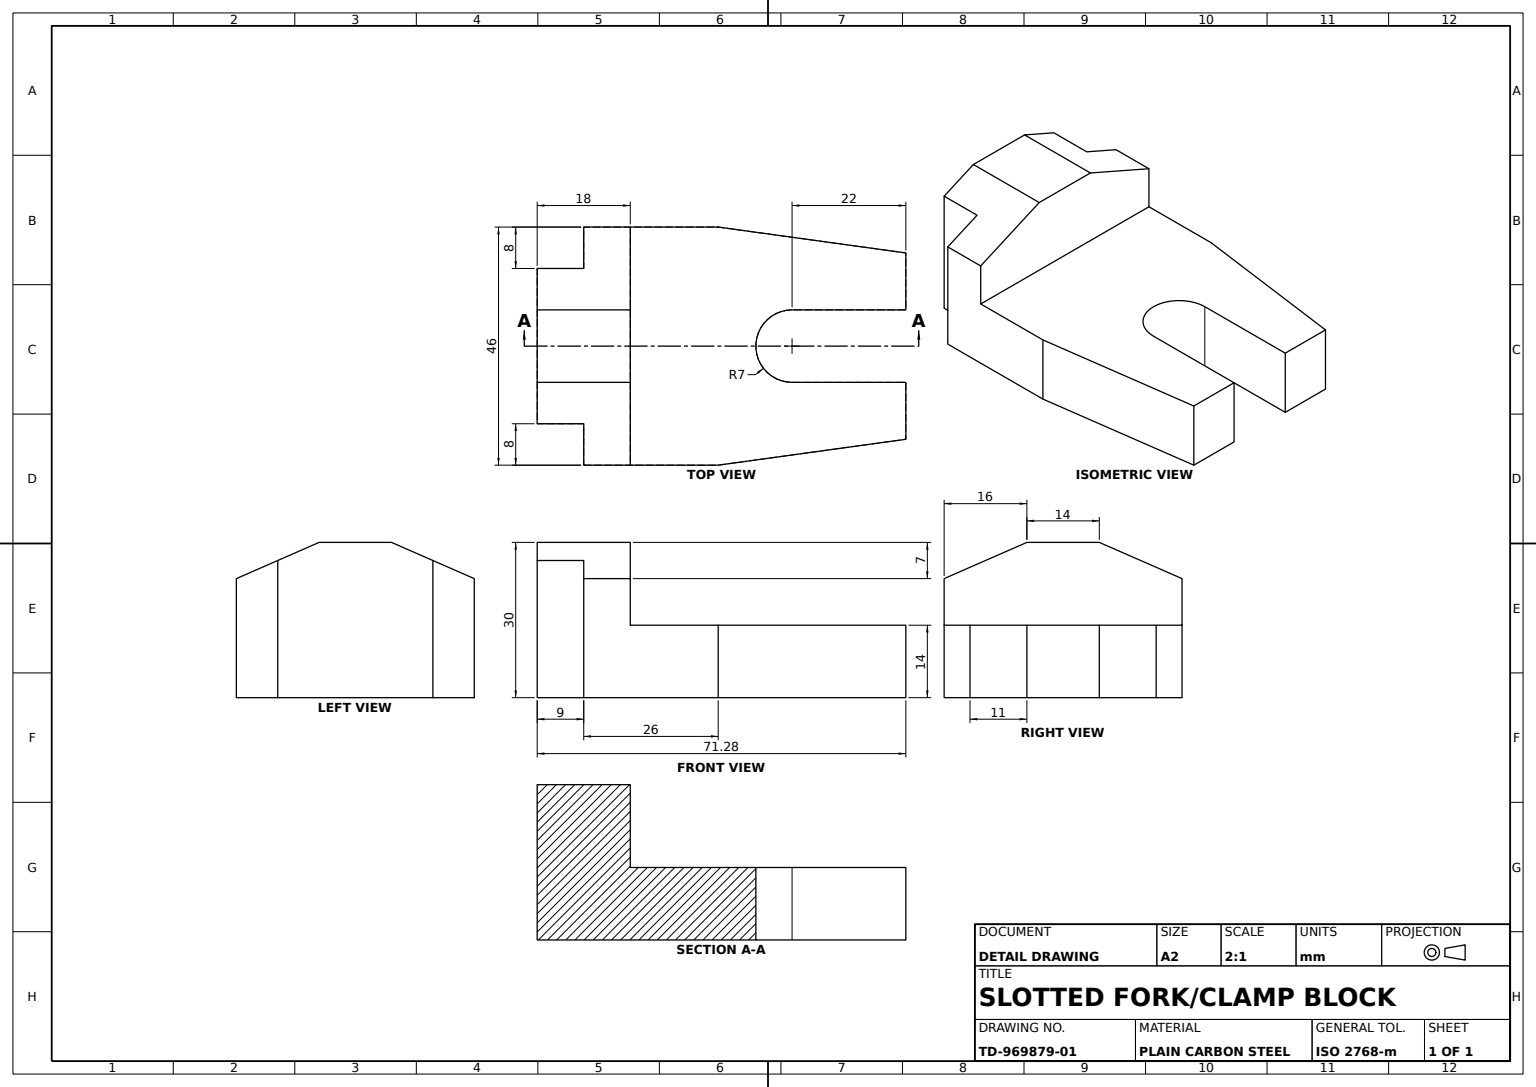
from build123d import *

# Parameters (mm, degrees)
BASE_PLATE_14MM_WITH_U_SLOT_DEPTH = 7
RAISED_BLOCK_18MM_DEPTH           = 9
STEP_CUT_SKETCH_W                 = 9
STEP_CUT_SKETCH_H                 = 8
STEP_CUT_DEPTH                    = 73.855407245


with BuildPart() as part:
    # Base Plate Profile Sketch → Base Plate 14mm with U-Slot (new, symmetric)
    with BuildSketch(Plane(origin=(0, 0, 0), x_dir=(1, 0, 0), z_dir=(0, 1, 0))):
        with BuildLine():
            Line((0, 23), (0, -23))
            Line((0, -23), (26, -23))
            Line((26, -23), (62.280898876, -18))
            Line((62.280898876, -18), (62.280898876, -7))
            Line((62.280898876, -7), (40.280898876, -7))
            ThreePointArc((40.280898876, -7), (33.280898876, 0), (40.280898876, 7))
            Line((40.280898876, 7), (62.280898876, 7))
            Line((62.280898876, 7), (62.280898876, 18))
            Line((62.280898876, 18), (26, 23))
            Line((26, 23), (0, 23))
        make_face()
    extrude(amount=BASE_PLATE_14MM_WITH_U_SLOT_DEPTH, both=True)

    # Raised Block Sketch → Raised Block 18mm (add, symmetric)
    with BuildSketch(Plane.ZY):
        Polygon((-23, 7), (-23, 16), (-7, 23), (7, 23), (23, 16), (23, 7), (23, -7), (-23, -7), align=None)
    extrude(amount=RAISED_BLOCK_18MM_DEPTH, both=True)

    # Step Cut Sketch → Step Cut (cut, through all)
    with BuildSketch(Plane(origin=(0, 23, 0), x_dir=(1, 0, 0), z_dir=(0, 1, 0))):
        with Locations((-4.5, 19)):
            Rectangle(STEP_CUT_SKETCH_W, STEP_CUT_SKETCH_H)
        with Locations((-4.5, -19)):
            Rectangle(STEP_CUT_SKETCH_W, STEP_CUT_SKETCH_H)
    extrude(amount=-STEP_CUT_DEPTH, mode=Mode.SUBTRACT)


solid = part.part
